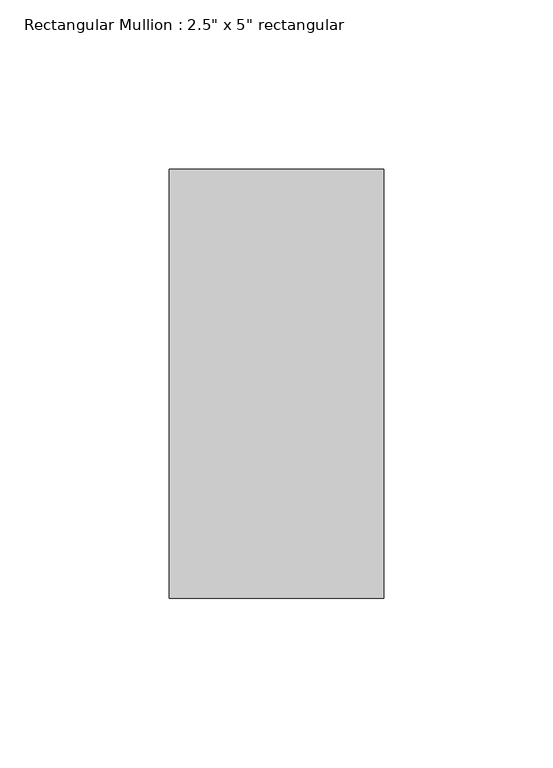
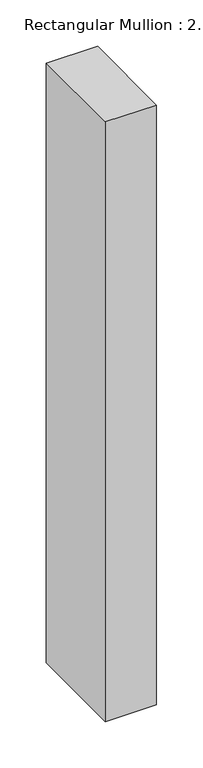
"""IFC4 building model written with IfcOpenShell, lengths in millimetres: member geometry."""

from ifc_helpers import new_model, si_unit, frame, origin, place, context, project, spatial, polyline, outline, extrude, source, transform, mapped, element, save


def member_2944fbe8(model_context):
    return source(origin(), model_context, "Body", "SweptSolid", [
        extrude(outline(polyline([(0.0, 63.5), (0.0, -63.5), (-63.5, -63.5), (-63.5, 63.5), (0.0, 63.5)])), frame((0.0, 0.0, -788.2127727), z_axis=(0.0, 0.0, 1.0), x_axis=(1.0, 0.0, 0.0)), (0.0, 0.0, 1.0), 788.2127727),
    ])


if __name__ == "__main__":
    model = new_model("IFC4")
    model_context = context("Model", 3, world=origin())
    ifc_project = project(units=[si_unit("LENGTHUNIT", "METRE", prefix="MILLI")], contexts=[model_context])
    site = spatial("IfcSite", under=ifc_project)
    building = spatial("IfcBuilding", under=site)
    placement = place(None, origin())
    member_shape = member_2944fbe8(model_context)
    element("IfcMember", 1, ObjectType="Rectangular Mullion : 2.5\" x 5\" rectangular", at=placement, inside=building, context=model_context, shape_type="MappedRepresentation", body=[
        mapped(member_shape, transform((0.0, 0.0, 0.0), x_axis=(1.0, 0.0, 0.0), y_axis=(0.0, 1.0, 0.0), z_axis=(0.0, 0.0, 1.0))),
    ])
    save(model, "model.ifc")

# Revit data of these elements
# Type "Rectangular Mullion : 2.5\" x 5\" rectangular"
#   built-in parameter 1007304 = 0.416667 (stored number, unit not read)
#   built-in parameter 1007301 = 0.104167 (stored number, unit not read)
#   built-in parameter 1007300 = 0.104167 (stored number, unit not read)
# Element 1 (IfcMember, "Rectangular Mullion : 2.5\" x 5\" rectangular")
#   Materials on its faces: "Aluminum"
# Materials
#   "Aluminum": class "Metal", colour RGB 247 247 247, transparency 0, Description = "Aluminum 6061", Cost = 0
